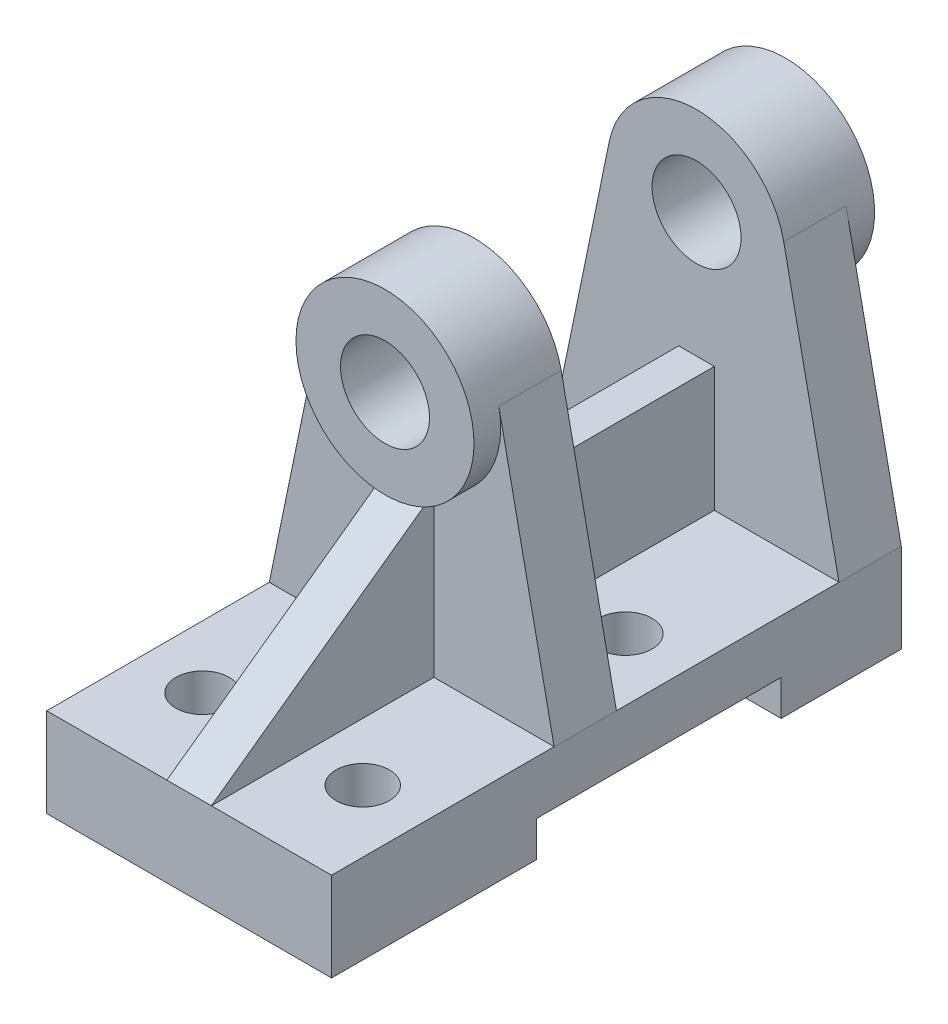
ISO-10303-21;
HEADER;
FILE_DESCRIPTION(('STEP AP214'),'2;1');
FILE_NAME('part.step','',(''),(''),'','','');
FILE_SCHEMA(('AUTOMOTIVE_DESIGN { 1 0 10303 214 1 1 1 1 }'));
ENDSEC;
DATA;
#1=APPLICATION_CONTEXT('core data for automotive mechanical design processes');
#2=APPLICATION_PROTOCOL_DEFINITION('international standard','automotive_design',2000,#1);
#3=PRODUCT_CONTEXT('',#1,'mechanical');
#4=PRODUCT('Part','Part','',(#3));
#5=PRODUCT_RELATED_PRODUCT_CATEGORY('part','',(#4));
#6=PRODUCT_DEFINITION_FORMATION('','',#4);
#7=PRODUCT_DEFINITION_CONTEXT('part definition',#1,'design');
#8=PRODUCT_DEFINITION('design','',#6,#7);
#9=PRODUCT_DEFINITION_SHAPE('','',#8);
#10=(LENGTH_UNIT() NAMED_UNIT(*) SI_UNIT(.MILLI.,.METRE.));
#11=(NAMED_UNIT(*) PLANE_ANGLE_UNIT() SI_UNIT($,.RADIAN.));
#12=(NAMED_UNIT(*) SI_UNIT($,.STERADIAN.) SOLID_ANGLE_UNIT());
#13=UNCERTAINTY_MEASURE_WITH_UNIT(LENGTH_MEASURE(1.E-05),#10,'distance_accuracy_value','');
#14=(GEOMETRIC_REPRESENTATION_CONTEXT(3) GLOBAL_UNCERTAINTY_ASSIGNED_CONTEXT((#13)) GLOBAL_UNIT_ASSIGNED_CONTEXT((#10,
#11,#12)) REPRESENTATION_CONTEXT('',''));
#15=CARTESIAN_POINT('',(0.,0.,0.));
#16=DIRECTION('',(0.,0.,1.));
#17=DIRECTION('',(1.,0.,0.));
#18=AXIS2_PLACEMENT_3D('',#15,#16,#17);
#19=CARTESIAN_POINT('',(32.,20.,0.));
#20=DIRECTION('',(0.,-1.,0.));
#21=DIRECTION('',(0.,0.,-1.));
#22=AXIS2_PLACEMENT_3D('',#19,#20,#21);
#23=PLANE('',#22);
#24=CARTESIAN_POINT('',(-18.,20.,107.));
#25=DIRECTION('',(0.,1.,0.));
#26=DIRECTION('',(0.,0.,1.));
#27=AXIS2_PLACEMENT_3D('',#24,#25,#26);
#28=CIRCLE('',#27,6.00000000000001);
#29=CARTESIAN_POINT('',(-18.,20.,113.));
#30=VERTEX_POINT('',#29);
#31=EDGE_CURVE('E600',#30,#30,#28,.T.);
#32=ORIENTED_EDGE('',*,*,#31,.F.);
#33=EDGE_LOOP('',(#32));
#34=FACE_BOUND('',#33,.T.);
#35=DIRECTION('',(0.,0.,1.));
#36=VECTOR('',#35,1.);
#37=CARTESIAN_POINT('',(-5.,20.,0.));
#38=LINE('',#37,#36);
#39=CARTESIAN_POINT('',(-5.,20.,78.));
#40=VERTEX_POINT('',#39);
#41=CARTESIAN_POINT('',(-5.,20.,128.));
#42=VERTEX_POINT('',#41);
#43=EDGE_CURVE('E215',#40,#42,#38,.T.);
#44=ORIENTED_EDGE('',*,*,#43,.F.);
#45=DIRECTION('',(1.,0.,0.));
#46=VECTOR('',#45,1.);
#47=CARTESIAN_POINT('',(0.,20.,78.));
#48=LINE('',#47,#46);
#49=CARTESIAN_POINT('',(-32.,20.,78.));
#50=VERTEX_POINT('',#49);
#51=EDGE_CURVE('E298',#50,#40,#48,.T.);
#52=ORIENTED_EDGE('',*,*,#51,.F.);
#53=DIRECTION('',(0.,0.,1.));
#54=VECTOR('',#53,1.);
#55=CARTESIAN_POINT('',(-32.,20.,0.));
#56=LINE('',#55,#54);
#57=CARTESIAN_POINT('',(-32.,20.,128.));
#58=VERTEX_POINT('',#57);
#59=EDGE_CURVE('E234',#50,#58,#56,.T.);
#60=ORIENTED_EDGE('',*,*,#59,.T.);
#61=DIRECTION('',(-1.,0.,0.));
#62=VECTOR('',#61,1.);
#63=CARTESIAN_POINT('',(32.,20.,128.));
#64=LINE('',#63,#62);
#65=EDGE_CURVE('E231',#42,#58,#64,.T.);
#66=ORIENTED_EDGE('',*,*,#65,.F.);
#67=EDGE_LOOP('',(#44,#52,#60,#66));
#68=FACE_BOUND('',#67,.T.);
#69=ADVANCED_FACE('F56',(#34,#68),#23,.F.);
#70=CARTESIAN_POINT('',(0.,0.,78.));
#71=DIRECTION('',(0.,0.,1.));
#72=DIRECTION('',(-1.,0.,0.));
#73=AXIS2_PLACEMENT_3D('',#70,#71,#72);
#74=PLANE('',#73);
#75=DIRECTION('',(0.,1.,0.));
#76=VECTOR('',#75,1.);
#77=CARTESIAN_POINT('',(5.,0.,78.));
#78=LINE('',#77,#76);
#79=CARTESIAN_POINT('',(5.,20.,78.));
#80=VERTEX_POINT('',#79);
#81=CARTESIAN_POINT('',(5.,56.,78.));
#82=VERTEX_POINT('',#81);
#83=EDGE_CURVE('E12',#80,#82,#78,.T.);
#84=ORIENTED_EDGE('',*,*,#83,.F.);
#85=CARTESIAN_POINT('',(32.,20.,78.));
#86=VERTEX_POINT('',#85);
#87=EDGE_CURVE('E294',#80,#86,#48,.T.);
#88=ORIENTED_EDGE('',*,*,#87,.T.);
#89=DIRECTION('',(0.202452606669412,-0.979292061671471,0.));
#90=VECTOR('',#89,1.);
#91=CARTESIAN_POINT('',(34.6536187572094,7.16406853737846,78.));
#92=LINE('',#91,#90);
#93=CARTESIAN_POINT('',(19.5858412334294,80.0490521333882,78.));
#94=VERTEX_POINT('',#93);
#95=EDGE_CURVE('E283',#94,#86,#92,.T.);
#96=ORIENTED_EDGE('',*,*,#95,.F.);
#97=CARTESIAN_POINT('',(0.,76.,78.));
#98=DIRECTION('',(0.,0.,1.));
#99=DIRECTION('',(1.,0.,0.));
#100=AXIS2_PLACEMENT_3D('',#97,#98,#99);
#101=CIRCLE('',#100,20.);
#102=CARTESIAN_POINT('',(0.,56.,78.));
#103=VERTEX_POINT('',#102);
#104=EDGE_CURVE('E318',#103,#94,#101,.T.);
#105=ORIENTED_EDGE('',*,*,#104,.F.);
#106=DIRECTION('',(1.,0.,0.));
#107=VECTOR('',#106,1.);
#108=CARTESIAN_POINT('',(0.,56.,78.));
#109=LINE('',#108,#107);
#110=EDGE_CURVE('E67',#82,#103,#109,.F.);
#111=ORIENTED_EDGE('',*,*,#110,.F.);
#112=EDGE_LOOP('',(#84,#88,#96,#105,#111));
#113=FACE_BOUND('',#112,.T.);
#114=ADVANCED_FACE('F430',(#113),#74,.T.);
#115=CARTESIAN_POINT('',(-18.,20.,48.));
#116=DIRECTION('',(0.,1.,0.));
#117=DIRECTION('',(0.,0.,1.));
#118=AXIS2_PLACEMENT_3D('',#115,#116,#117);
#119=CIRCLE('',#118,6.);
#120=CARTESIAN_POINT('',(-18.,20.,54.));
#121=VERTEX_POINT('',#120);
#122=EDGE_CURVE('E407',#121,#121,#119,.T.);
#123=ORIENTED_EDGE('',*,*,#122,.F.);
#124=EDGE_LOOP('',(#123));
#125=FACE_BOUND('',#124,.T.);
#126=DIRECTION('',(0.,0.,1.));
#127=VECTOR('',#126,1.);
#128=CARTESIAN_POINT('',(-4.00000000000001,20.,14.));
#129=LINE('',#128,#127);
#130=CARTESIAN_POINT('',(-4.00000000000001,20.,14.));
#131=VERTEX_POINT('',#130);
#132=CARTESIAN_POINT('',(-4.,20.,64.));
#133=VERTEX_POINT('',#132);
#134=EDGE_CURVE('E244',#131,#133,#129,.T.);
#135=ORIENTED_EDGE('',*,*,#134,.F.);
#136=DIRECTION('',(1.,0.,0.));
#137=VECTOR('',#136,1.);
#138=CARTESIAN_POINT('',(0.,20.,14.));
#139=LINE('',#138,#137);
#140=CARTESIAN_POINT('',(-32.,20.,14.));
#141=VERTEX_POINT('',#140);
#142=EDGE_CURVE('E333',#141,#131,#139,.T.);
#143=ORIENTED_EDGE('',*,*,#142,.F.);
#144=CARTESIAN_POINT('',(-32.,20.,64.));
#145=VERTEX_POINT('',#144);
#146=EDGE_CURVE('E372',#141,#145,#56,.T.);
#147=ORIENTED_EDGE('',*,*,#146,.T.);
#148=DIRECTION('',(1.,0.,0.));
#149=VECTOR('',#148,1.);
#150=CARTESIAN_POINT('',(0.,20.,64.));
#151=LINE('',#150,#149);
#152=EDGE_CURVE('E284',#145,#133,#151,.T.);
#153=ORIENTED_EDGE('',*,*,#152,.T.);
#154=EDGE_LOOP('',(#135,#143,#147,#153));
#155=FACE_BOUND('',#154,.T.);
#156=ADVANCED_FACE('F446',(#125,#155),#23,.F.);
#157=CARTESIAN_POINT('',(18.,20.,48.));
#158=DIRECTION('',(0.,1.,0.));
#159=DIRECTION('',(0.,0.,1.));
#160=AXIS2_PLACEMENT_3D('',#157,#158,#159);
#161=CIRCLE('',#160,6.);
#162=CARTESIAN_POINT('',(18.,20.,54.));
#163=VERTEX_POINT('',#162);
#164=EDGE_CURVE('E413',#163,#163,#161,.T.);
#165=ORIENTED_EDGE('',*,*,#164,.F.);
#166=EDGE_LOOP('',(#165));
#167=FACE_BOUND('',#166,.T.);
#168=DIRECTION('',(0.,0.,1.));
#169=VECTOR('',#168,1.);
#170=CARTESIAN_POINT('',(32.,20.,0.));
#171=LINE('',#170,#169);
#172=CARTESIAN_POINT('',(32.,20.,14.));
#173=VERTEX_POINT('',#172);
#174=CARTESIAN_POINT('',(32.,20.,64.));
#175=VERTEX_POINT('',#174);
#176=EDGE_CURVE('E354',#173,#175,#171,.T.);
#177=ORIENTED_EDGE('',*,*,#176,.F.);
#178=CARTESIAN_POINT('',(4.00000000000001,20.,14.));
#179=VERTEX_POINT('',#178);
#180=EDGE_CURVE('E326',#179,#173,#139,.T.);
#181=ORIENTED_EDGE('',*,*,#180,.F.);
#182=DIRECTION('',(0.,0.,-1.));
#183=VECTOR('',#182,1.);
#184=CARTESIAN_POINT('',(4.00000000000001,20.,14.));
#185=LINE('',#184,#183);
#186=CARTESIAN_POINT('',(4.,20.,64.));
#187=VERTEX_POINT('',#186);
#188=EDGE_CURVE('E250',#187,#179,#185,.T.);
#189=ORIENTED_EDGE('',*,*,#188,.F.);
#190=EDGE_CURVE('E278',#187,#175,#151,.T.);
#191=ORIENTED_EDGE('',*,*,#190,.T.);
#192=EDGE_LOOP('',(#177,#181,#189,#191));
#193=FACE_BOUND('',#192,.T.);
#194=ADVANCED_FACE('F490',(#167,#193),#23,.F.);
#195=CARTESIAN_POINT('',(0.,0.,14.));
#196=DIRECTION('',(0.,0.,-1.));
#197=DIRECTION('',(-1.,0.,0.));
#198=AXIS2_PLACEMENT_3D('',#195,#196,#197);
#199=PLANE('',#198);
#200=CARTESIAN_POINT('',(0.,76.,14.));
#201=DIRECTION('',(0.,0.,-1.));
#202=DIRECTION('',(-1.,0.,0.));
#203=AXIS2_PLACEMENT_3D('',#200,#201,#202);
#204=CIRCLE('',#203,10.);
#205=CARTESIAN_POINT('',(-10.,76.,14.));
#206=VERTEX_POINT('',#205);
#207=EDGE_CURVE('E331',#206,#206,#204,.T.);
#208=ORIENTED_EDGE('',*,*,#207,.T.);
#209=EDGE_LOOP('',(#208));
#210=FACE_BOUND('',#209,.T.);
#211=DIRECTION('',(0.202452606669412,-0.979292061671471,0.));
#212=VECTOR('',#211,1.);
#213=CARTESIAN_POINT('',(34.6536187572094,7.16406853737846,14.));
#214=LINE('',#213,#212);
#215=CARTESIAN_POINT('',(19.5858412334294,80.0490521333882,14.));
#216=VERTEX_POINT('',#215);
#217=EDGE_CURVE('E329',#216,#173,#214,.T.);
#218=ORIENTED_EDGE('',*,*,#217,.F.);
#219=CARTESIAN_POINT('',(0.,76.,14.));
#220=DIRECTION('',(0.,0.,-1.));
#221=DIRECTION('',(-1.,0.,0.));
#222=AXIS2_PLACEMENT_3D('',#219,#220,#221);
#223=CIRCLE('',#222,20.);
#224=CARTESIAN_POINT('',(-19.5858412334294,80.0490521333882,14.));
#225=VERTEX_POINT('',#224);
#226=EDGE_CURVE('E321',#225,#216,#223,.T.);
#227=ORIENTED_EDGE('',*,*,#226,.F.);
#228=DIRECTION('',(-0.202452606669412,-0.979292061671471,0.));
#229=VECTOR('',#228,1.);
#230=CARTESIAN_POINT('',(-34.6536187572094,7.16406853737846,14.));
#231=LINE('',#230,#229);
#232=EDGE_CURVE('E322',#225,#141,#231,.T.);
#233=ORIENTED_EDGE('',*,*,#232,.T.);
#234=ORIENTED_EDGE('',*,*,#142,.T.);
#235=DIRECTION('',(0.,-1.,0.));
#236=VECTOR('',#235,1.);
#237=CARTESIAN_POINT('',(-4.00000000000001,48.,14.));
#238=LINE('',#237,#236);
#239=CARTESIAN_POINT('',(-4.00000000000001,48.,14.));
#240=VERTEX_POINT('',#239);
#241=EDGE_CURVE('E256',#240,#131,#238,.T.);
#242=ORIENTED_EDGE('',*,*,#241,.F.);
#243=DIRECTION('',(-1.,0.,0.));
#244=VECTOR('',#243,1.);
#245=CARTESIAN_POINT('',(-4.00000000000001,48.,14.));
#246=LINE('',#245,#244);
#247=CARTESIAN_POINT('',(4.00000000000001,48.,14.));
#248=VERTEX_POINT('',#247);
#249=EDGE_CURVE('E259',#248,#240,#246,.T.);
#250=ORIENTED_EDGE('',*,*,#249,.F.);
#251=DIRECTION('',(0.,-1.,0.));
#252=VECTOR('',#251,1.);
#253=CARTESIAN_POINT('',(4.00000000000001,48.,14.));
#254=LINE('',#253,#252);
#255=EDGE_CURVE('E265',#248,#179,#254,.T.);
#256=ORIENTED_EDGE('',*,*,#255,.T.);
#257=ORIENTED_EDGE('',*,*,#180,.T.);
#258=EDGE_LOOP('',(#218,#227,#233,#234,#242,#250,#256,#257));
#259=FACE_BOUND('',#258,.T.);
#260=ADVANCED_FACE('F470',(#210,#259),#199,.F.);
#261=CARTESIAN_POINT('',(0.,0.,64.));
#262=DIRECTION('',(0.,0.,1.));
#263=DIRECTION('',(-1.,0.,0.));
#264=AXIS2_PLACEMENT_3D('',#261,#262,#263);
#265=PLANE('',#264);
#266=CARTESIAN_POINT('',(0.,76.,64.));
#267=DIRECTION('',(0.,0.,-1.));
#268=DIRECTION('',(-1.,0.,0.));
#269=AXIS2_PLACEMENT_3D('',#266,#267,#268);
#270=CIRCLE('',#269,10.);
#271=CARTESIAN_POINT('',(-10.,76.,64.));
#272=VERTEX_POINT('',#271);
#273=EDGE_CURVE('E287',#272,#272,#270,.T.);
#274=ORIENTED_EDGE('',*,*,#273,.F.);
#275=EDGE_LOOP('',(#274));
#276=FACE_BOUND('',#275,.T.);
#277=DIRECTION('',(0.202452606669412,-0.979292061671471,0.));
#278=VECTOR('',#277,1.);
#279=CARTESIAN_POINT('',(34.6536187572094,7.16406853737846,64.));
#280=LINE('',#279,#278);
#281=CARTESIAN_POINT('',(19.5858412334294,80.0490521333882,64.));
#282=VERTEX_POINT('',#281);
#283=EDGE_CURVE('E285',#282,#175,#280,.T.);
#284=ORIENTED_EDGE('',*,*,#283,.T.);
#285=ORIENTED_EDGE('',*,*,#190,.F.);
#286=DIRECTION('',(0.,-1.,0.));
#287=VECTOR('',#286,1.);
#288=CARTESIAN_POINT('',(4.,48.,64.));
#289=LINE('',#288,#287);
#290=CARTESIAN_POINT('',(4.,48.,64.));
#291=VERTEX_POINT('',#290);
#292=EDGE_CURVE('E270',#291,#187,#289,.T.);
#293=ORIENTED_EDGE('',*,*,#292,.F.);
#294=DIRECTION('',(1.,0.,0.));
#295=VECTOR('',#294,1.);
#296=CARTESIAN_POINT('',(-4.,48.,64.));
#297=LINE('',#296,#295);
#298=CARTESIAN_POINT('',(-4.00000000000001,48.,64.));
#299=VERTEX_POINT('',#298);
#300=EDGE_CURVE('E251',#299,#291,#297,.T.);
#301=ORIENTED_EDGE('',*,*,#300,.F.);
#302=DIRECTION('',(0.,-1.,0.));
#303=VECTOR('',#302,1.);
#304=CARTESIAN_POINT('',(-4.,48.,64.));
#305=LINE('',#304,#303);
#306=EDGE_CURVE('E81',#299,#133,#305,.T.);
#307=ORIENTED_EDGE('',*,*,#306,.T.);
#308=ORIENTED_EDGE('',*,*,#152,.F.);
#309=DIRECTION('',(-0.202452606669412,-0.979292061671471,0.));
#310=VECTOR('',#309,1.);
#311=CARTESIAN_POINT('',(-34.6536187572094,7.16406853737846,64.));
#312=LINE('',#311,#310);
#313=CARTESIAN_POINT('',(-19.5858412334294,80.0490521333882,64.));
#314=VERTEX_POINT('',#313);
#315=EDGE_CURVE('E280',#314,#145,#312,.T.);
#316=ORIENTED_EDGE('',*,*,#315,.F.);
#317=CARTESIAN_POINT('',(0.,76.,64.));
#318=DIRECTION('',(0.,0.,-1.));
#319=DIRECTION('',(-1.,0.,0.));
#320=AXIS2_PLACEMENT_3D('',#317,#318,#319);
#321=CIRCLE('',#320,20.);
#322=EDGE_CURVE('E290',#314,#282,#321,.T.);
#323=ORIENTED_EDGE('',*,*,#322,.T.);
#324=EDGE_LOOP('',(#284,#285,#293,#301,#307,#308,#316,#323));
#325=FACE_BOUND('',#324,.T.);
#326=ADVANCED_FACE('F452',(#276,#325),#265,.F.);
#327=CARTESIAN_POINT('',(18.,20.,107.));
#328=DIRECTION('',(0.,1.,0.));
#329=DIRECTION('',(0.,0.,1.));
#330=AXIS2_PLACEMENT_3D('',#327,#328,#329);
#331=CIRCLE('',#330,6.);
#332=CARTESIAN_POINT('',(18.,20.,113.));
#333=VERTEX_POINT('',#332);
#334=EDGE_CURVE('E418',#333,#333,#331,.T.);
#335=ORIENTED_EDGE('',*,*,#334,.F.);
#336=EDGE_LOOP('',(#335));
#337=FACE_BOUND('',#336,.T.);
#338=ORIENTED_EDGE('',*,*,#87,.F.);
#339=DIRECTION('',(0.,0.,1.));
#340=VECTOR('',#339,1.);
#341=CARTESIAN_POINT('',(5.,20.,0.));
#342=LINE('',#341,#340);
#343=CARTESIAN_POINT('',(5.,20.,128.));
#344=VERTEX_POINT('',#343);
#345=EDGE_CURVE('E216',#80,#344,#342,.T.);
#346=ORIENTED_EDGE('',*,*,#345,.T.);
#347=CARTESIAN_POINT('',(32.,20.,128.));
#348=VERTEX_POINT('',#347);
#349=EDGE_CURVE('E238',#348,#344,#64,.T.);
#350=ORIENTED_EDGE('',*,*,#349,.F.);
#351=EDGE_CURVE('E350',#86,#348,#171,.T.);
#352=ORIENTED_EDGE('',*,*,#351,.F.);
#353=EDGE_LOOP('',(#338,#346,#350,#352));
#354=FACE_BOUND('',#353,.T.);
#355=ADVANCED_FACE('F483',(#337,#354),#23,.F.);
#356=CARTESIAN_POINT('',(32.,0.,0.));
#357=DIRECTION('',(0.,0.,1.));
#358=DIRECTION('',(1.,0.,0.));
#359=AXIS2_PLACEMENT_3D('',#356,#357,#358);
#360=PLANE('',#359);
#361=DIRECTION('',(-1.,0.,0.));
#362=VECTOR('',#361,1.);
#363=CARTESIAN_POINT('',(32.,0.,0.));
#364=LINE('',#363,#362);
#365=CARTESIAN_POINT('',(32.,0.,0.));
#366=VERTEX_POINT('',#365);
#367=CARTESIAN_POINT('',(-32.,0.,0.));
#368=VERTEX_POINT('',#367);
#369=EDGE_CURVE('E370',#366,#368,#364,.T.);
#370=ORIENTED_EDGE('',*,*,#369,.T.);
#371=DIRECTION('',(0.,1.,0.));
#372=VECTOR('',#371,1.);
#373=CARTESIAN_POINT('',(-32.,0.,0.));
#374=LINE('',#373,#372);
#375=CARTESIAN_POINT('',(-32.,20.,0.));
#376=VERTEX_POINT('',#375);
#377=EDGE_CURVE('E341',#368,#376,#374,.T.);
#378=ORIENTED_EDGE('',*,*,#377,.T.);
#379=DIRECTION('',(-0.202452606669412,-0.979292061671471,0.));
#380=VECTOR('',#379,1.);
#381=CARTESIAN_POINT('',(-34.6536187572094,7.16406853737846,0.));
#382=LINE('',#381,#380);
#383=CARTESIAN_POINT('',(-19.5858412334294,80.0490521333882,0.));
#384=VERTEX_POINT('',#383);
#385=EDGE_CURVE('E320',#384,#376,#382,.T.);
#386=ORIENTED_EDGE('',*,*,#385,.F.);
#387=CARTESIAN_POINT('',(0.,76.,0.));
#388=DIRECTION('',(0.,0.,-1.));
#389=DIRECTION('',(-1.,0.,0.));
#390=AXIS2_PLACEMENT_3D('',#387,#388,#389);
#391=CIRCLE('',#390,20.);
#392=CARTESIAN_POINT('',(19.5858412334294,80.0490521333882,0.));
#393=VERTEX_POINT('',#392);
#394=EDGE_CURVE('E319',#393,#384,#391,.T.);
#395=ORIENTED_EDGE('',*,*,#394,.F.);
#396=DIRECTION('',(0.202452606669412,-0.979292061671471,0.));
#397=VECTOR('',#396,1.);
#398=CARTESIAN_POINT('',(34.6536187572094,7.16406853737846,0.));
#399=LINE('',#398,#397);
#400=CARTESIAN_POINT('',(32.,20.,0.));
#401=VERTEX_POINT('',#400);
#402=EDGE_CURVE('E323',#393,#401,#399,.T.);
#403=ORIENTED_EDGE('',*,*,#402,.T.);
#404=DIRECTION('',(0.,1.,0.));
#405=VECTOR('',#404,1.);
#406=CARTESIAN_POINT('',(32.,0.,0.));
#407=LINE('',#406,#405);
#408=EDGE_CURVE('E349',#366,#401,#407,.T.);
#409=ORIENTED_EDGE('',*,*,#408,.F.);
#410=EDGE_LOOP('',(#370,#378,#386,#395,#403,#409));
#411=FACE_BOUND('',#410,.T.);
#412=ADVANCED_FACE('F62',(#411),#360,.F.);
#413=CARTESIAN_POINT('',(32.,0.,128.));
#414=DIRECTION('',(0.,0.,-1.));
#415=DIRECTION('',(-1.,0.,0.));
#416=AXIS2_PLACEMENT_3D('',#413,#414,#415);
#417=PLANE('',#416);
#418=ORIENTED_EDGE('',*,*,#349,.T.);
#419=DIRECTION('',(-1.,0.,0.));
#420=VECTOR('',#419,1.);
#421=CARTESIAN_POINT('',(32.,20.,128.));
#422=LINE('',#421,#420);
#423=EDGE_CURVE('E227',#42,#344,#422,.F.);
#424=ORIENTED_EDGE('',*,*,#423,.F.);
#425=ORIENTED_EDGE('',*,*,#65,.T.);
#426=DIRECTION('',(0.,-1.,0.));
#427=VECTOR('',#426,1.);
#428=CARTESIAN_POINT('',(-32.,0.,128.));
#429=LINE('',#428,#427);
#430=CARTESIAN_POINT('',(-32.,0.,128.));
#431=VERTEX_POINT('',#430);
#432=EDGE_CURVE('E373',#58,#431,#429,.T.);
#433=ORIENTED_EDGE('',*,*,#432,.T.);
#434=DIRECTION('',(-1.,0.,0.));
#435=VECTOR('',#434,1.);
#436=CARTESIAN_POINT('',(32.,0.,128.));
#437=LINE('',#436,#435);
#438=CARTESIAN_POINT('',(32.,0.,128.));
#439=VERTEX_POINT('',#438);
#440=EDGE_CURVE('E237',#439,#431,#437,.T.);
#441=ORIENTED_EDGE('',*,*,#440,.F.);
#442=DIRECTION('',(0.,-1.,0.));
#443=VECTOR('',#442,1.);
#444=CARTESIAN_POINT('',(32.,0.,128.));
#445=LINE('',#444,#443);
#446=EDGE_CURVE('E352',#348,#439,#445,.T.);
#447=ORIENTED_EDGE('',*,*,#446,.F.);
#448=EDGE_LOOP('',(#418,#424,#425,#433,#441,#447));
#449=FACE_BOUND('',#448,.T.);
#450=ADVANCED_FACE('F245',(#449),#417,.F.);
#451=CARTESIAN_POINT('',(32.,0.,82.));
#452=DIRECTION('',(0.,1.,0.));
#453=DIRECTION('',(0.,0.,1.));
#454=AXIS2_PLACEMENT_3D('',#451,#452,#453);
#455=PLANE('',#454);
#456=CARTESIAN_POINT('',(-18.,0.,107.));
#457=DIRECTION('',(0.,1.,0.));
#458=DIRECTION('',(0.,0.,1.));
#459=AXIS2_PLACEMENT_3D('',#456,#457,#458);
#460=CIRCLE('',#459,6.00000000000001);
#461=CARTESIAN_POINT('',(-18.,0.,113.));
#462=VERTEX_POINT('',#461);
#463=EDGE_CURVE('E419',#462,#462,#460,.T.);
#464=ORIENTED_EDGE('',*,*,#463,.T.);
#465=EDGE_LOOP('',(#464));
#466=FACE_BOUND('',#465,.T.);
#467=CARTESIAN_POINT('',(18.,0.,107.));
#468=DIRECTION('',(0.,1.,0.));
#469=DIRECTION('',(0.,0.,1.));
#470=AXIS2_PLACEMENT_3D('',#467,#468,#469);
#471=CIRCLE('',#470,6.);
#472=CARTESIAN_POINT('',(18.,0.,113.));
#473=VERTEX_POINT('',#472);
#474=EDGE_CURVE('E596',#473,#473,#471,.T.);
#475=ORIENTED_EDGE('',*,*,#474,.T.);
#476=EDGE_LOOP('',(#475));
#477=FACE_BOUND('',#476,.T.);
#478=ORIENTED_EDGE('',*,*,#440,.T.);
#479=DIRECTION('',(0.,0.,-1.));
#480=VECTOR('',#479,1.);
#481=CARTESIAN_POINT('',(-32.,0.,82.));
#482=LINE('',#481,#480);
#483=CARTESIAN_POINT('',(-32.,0.,82.));
#484=VERTEX_POINT('',#483);
#485=EDGE_CURVE('E376',#431,#484,#482,.T.);
#486=ORIENTED_EDGE('',*,*,#485,.T.);
#487=DIRECTION('',(-1.,0.,0.));
#488=VECTOR('',#487,1.);
#489=CARTESIAN_POINT('',(32.,0.,82.));
#490=LINE('',#489,#488);
#491=CARTESIAN_POINT('',(32.,0.,82.));
#492=VERTEX_POINT('',#491);
#493=EDGE_CURVE('E400',#492,#484,#490,.T.);
#494=ORIENTED_EDGE('',*,*,#493,.F.);
#495=DIRECTION('',(0.,0.,-1.));
#496=VECTOR('',#495,1.);
#497=CARTESIAN_POINT('',(32.,0.,82.));
#498=LINE('',#497,#496);
#499=EDGE_CURVE('E357',#439,#492,#498,.T.);
#500=ORIENTED_EDGE('',*,*,#499,.F.);
#501=EDGE_LOOP('',(#478,#486,#494,#500));
#502=FACE_BOUND('',#501,.T.);
#503=ADVANCED_FACE('F551',(#466,#477,#502),#455,.F.);
#504=CARTESIAN_POINT('',(32.,0.,82.));
#505=DIRECTION('',(0.,0.,1.));
#506=DIRECTION('',(0.,-1.,0.));
#507=AXIS2_PLACEMENT_3D('',#504,#505,#506);
#508=PLANE('',#507);
#509=ORIENTED_EDGE('',*,*,#493,.T.);
#510=DIRECTION('',(0.,1.,0.));
#511=VECTOR('',#510,1.);
#512=CARTESIAN_POINT('',(-32.,0.,82.));
#513=LINE('',#512,#511);
#514=CARTESIAN_POINT('',(-32.,7.99999999999999,82.));
#515=VERTEX_POINT('',#514);
#516=EDGE_CURVE('E378',#484,#515,#513,.T.);
#517=ORIENTED_EDGE('',*,*,#516,.T.);
#518=DIRECTION('',(-1.,0.,0.));
#519=VECTOR('',#518,1.);
#520=CARTESIAN_POINT('',(32.,7.99999999999999,82.));
#521=LINE('',#520,#519);
#522=CARTESIAN_POINT('',(32.,7.99999999999999,82.));
#523=VERTEX_POINT('',#522);
#524=EDGE_CURVE('E391',#523,#515,#521,.T.);
#525=ORIENTED_EDGE('',*,*,#524,.F.);
#526=DIRECTION('',(0.,1.,0.));
#527=VECTOR('',#526,1.);
#528=CARTESIAN_POINT('',(32.,0.,82.));
#529=LINE('',#528,#527);
#530=EDGE_CURVE('E360',#492,#523,#529,.T.);
#531=ORIENTED_EDGE('',*,*,#530,.F.);
#532=EDGE_LOOP('',(#509,#517,#525,#531));
#533=FACE_BOUND('',#532,.T.);
#534=ADVANCED_FACE('F546',(#533),#508,.F.);
#535=CARTESIAN_POINT('',(32.,8.,27.));
#536=DIRECTION('',(0.,1.,0.));
#537=DIRECTION('',(0.,0.,1.));
#538=AXIS2_PLACEMENT_3D('',#535,#536,#537);
#539=PLANE('',#538);
#540=CARTESIAN_POINT('',(18.,7.99999999999999,48.));
#541=DIRECTION('',(0.,1.,0.));
#542=DIRECTION('',(0.,0.,1.));
#543=AXIS2_PLACEMENT_3D('',#540,#541,#542);
#544=CIRCLE('',#543,6.);
#545=CARTESIAN_POINT('',(18.,7.99999999999999,54.));
#546=VERTEX_POINT('',#545);
#547=EDGE_CURVE('E64',#546,#546,#544,.T.);
#548=ORIENTED_EDGE('',*,*,#547,.T.);
#549=EDGE_LOOP('',(#548));
#550=FACE_BOUND('',#549,.T.);
#551=CARTESIAN_POINT('',(-18.,7.99999999999999,48.));
#552=DIRECTION('',(0.,1.,0.));
#553=DIRECTION('',(0.,0.,1.));
#554=AXIS2_PLACEMENT_3D('',#551,#552,#553);
#555=CIRCLE('',#554,6.);
#556=CARTESIAN_POINT('',(-18.,7.99999999999999,54.));
#557=VERTEX_POINT('',#556);
#558=EDGE_CURVE('E404',#557,#557,#555,.T.);
#559=ORIENTED_EDGE('',*,*,#558,.T.);
#560=EDGE_LOOP('',(#559));
#561=FACE_BOUND('',#560,.T.);
#562=ORIENTED_EDGE('',*,*,#524,.T.);
#563=DIRECTION('',(0.,0.,-1.));
#564=VECTOR('',#563,1.);
#565=CARTESIAN_POINT('',(-32.,8.,27.));
#566=LINE('',#565,#564);
#567=CARTESIAN_POINT('',(-32.,8.,27.));
#568=VERTEX_POINT('',#567);
#569=EDGE_CURVE('E385',#515,#568,#566,.T.);
#570=ORIENTED_EDGE('',*,*,#569,.T.);
#571=DIRECTION('',(-1.,0.,0.));
#572=VECTOR('',#571,1.);
#573=CARTESIAN_POINT('',(32.,8.,27.));
#574=LINE('',#573,#572);
#575=CARTESIAN_POINT('',(32.,8.,27.));
#576=VERTEX_POINT('',#575);
#577=EDGE_CURVE('E392',#576,#568,#574,.T.);
#578=ORIENTED_EDGE('',*,*,#577,.F.);
#579=DIRECTION('',(0.,0.,-1.));
#580=VECTOR('',#579,1.);
#581=CARTESIAN_POINT('',(32.,8.,27.));
#582=LINE('',#581,#580);
#583=EDGE_CURVE('E363',#523,#576,#582,.T.);
#584=ORIENTED_EDGE('',*,*,#583,.F.);
#585=EDGE_LOOP('',(#562,#570,#578,#584));
#586=FACE_BOUND('',#585,.T.);
#587=ADVANCED_FACE('F542',(#550,#561,#586),#539,.F.);
#588=CARTESIAN_POINT('',(32.,0.,27.));
#589=DIRECTION('',(0.,0.,-1.));
#590=DIRECTION('',(0.,1.,0.));
#591=AXIS2_PLACEMENT_3D('',#588,#589,#590);
#592=PLANE('',#591);
#593=ORIENTED_EDGE('',*,*,#577,.T.);
#594=DIRECTION('',(0.,-1.,0.));
#595=VECTOR('',#594,1.);
#596=CARTESIAN_POINT('',(-32.,0.,27.));
#597=LINE('',#596,#595);
#598=CARTESIAN_POINT('',(-32.,0.,27.));
#599=VERTEX_POINT('',#598);
#600=EDGE_CURVE('E383',#568,#599,#597,.T.);
#601=ORIENTED_EDGE('',*,*,#600,.T.);
#602=DIRECTION('',(-1.,0.,0.));
#603=VECTOR('',#602,1.);
#604=CARTESIAN_POINT('',(32.,0.,27.));
#605=LINE('',#604,#603);
#606=CARTESIAN_POINT('',(32.,0.,27.));
#607=VERTEX_POINT('',#606);
#608=EDGE_CURVE('E393',#607,#599,#605,.T.);
#609=ORIENTED_EDGE('',*,*,#608,.F.);
#610=DIRECTION('',(0.,-1.,0.));
#611=VECTOR('',#610,1.);
#612=CARTESIAN_POINT('',(32.,0.,27.));
#613=LINE('',#612,#611);
#614=EDGE_CURVE('E361',#576,#607,#613,.T.);
#615=ORIENTED_EDGE('',*,*,#614,.F.);
#616=EDGE_LOOP('',(#593,#601,#609,#615));
#617=FACE_BOUND('',#616,.T.);
#618=ADVANCED_FACE('F536',(#617),#592,.F.);
#619=CARTESIAN_POINT('',(32.,0.,0.));
#620=DIRECTION('',(0.,1.,0.));
#621=DIRECTION('',(0.,0.,1.));
#622=AXIS2_PLACEMENT_3D('',#619,#620,#621);
#623=PLANE('',#622);
#624=ORIENTED_EDGE('',*,*,#608,.T.);
#625=DIRECTION('',(0.,0.,-1.));
#626=VECTOR('',#625,1.);
#627=CARTESIAN_POINT('',(-32.,0.,0.));
#628=LINE('',#627,#626);
#629=EDGE_CURVE('E346',#599,#368,#628,.T.);
#630=ORIENTED_EDGE('',*,*,#629,.T.);
#631=ORIENTED_EDGE('',*,*,#369,.F.);
#632=DIRECTION('',(0.,0.,-1.));
#633=VECTOR('',#632,1.);
#634=CARTESIAN_POINT('',(32.,0.,0.));
#635=LINE('',#634,#633);
#636=EDGE_CURVE('E362',#607,#366,#635,.T.);
#637=ORIENTED_EDGE('',*,*,#636,.F.);
#638=EDGE_LOOP('',(#624,#630,#631,#637));
#639=FACE_BOUND('',#638,.T.);
#640=ADVANCED_FACE('F533',(#639),#623,.F.);
#641=CARTESIAN_POINT('',(32.,0.,0.));
#642=DIRECTION('',(1.,0.,0.));
#643=DIRECTION('',(0.,0.,-1.));
#644=AXIS2_PLACEMENT_3D('',#641,#642,#643);
#645=PLANE('',#644);
#646=ORIENTED_EDGE('',*,*,#408,.T.);
#647=EDGE_CURVE('E353',#401,#173,#171,.T.);
#648=ORIENTED_EDGE('',*,*,#647,.T.);
#649=ORIENTED_EDGE('',*,*,#176,.T.);
#650=DIRECTION('',(0.,0.,1.));
#651=VECTOR('',#650,1.);
#652=CARTESIAN_POINT('',(32.,20.,64.));
#653=LINE('',#652,#651);
#654=EDGE_CURVE('E310',#175,#86,#653,.T.);
#655=ORIENTED_EDGE('',*,*,#654,.T.);
#656=ORIENTED_EDGE('',*,*,#351,.T.);
#657=ORIENTED_EDGE('',*,*,#446,.T.);
#658=ORIENTED_EDGE('',*,*,#499,.T.);
#659=ORIENTED_EDGE('',*,*,#530,.T.);
#660=ORIENTED_EDGE('',*,*,#583,.T.);
#661=ORIENTED_EDGE('',*,*,#614,.T.);
#662=ORIENTED_EDGE('',*,*,#636,.T.);
#663=EDGE_LOOP('',(#646,#648,#649,#655,#656,#657,#658,#659,#660,#661,#662));
#664=FACE_BOUND('',#663,.T.);
#665=ADVANCED_FACE('F518',(#664),#645,.T.);
#666=CARTESIAN_POINT('',(-32.,0.,0.));
#667=DIRECTION('',(1.,0.,0.));
#668=DIRECTION('',(0.,0.,-1.));
#669=AXIS2_PLACEMENT_3D('',#666,#667,#668);
#670=PLANE('',#669);
#671=ORIENTED_EDGE('',*,*,#377,.F.);
#672=ORIENTED_EDGE('',*,*,#629,.F.);
#673=ORIENTED_EDGE('',*,*,#600,.F.);
#674=ORIENTED_EDGE('',*,*,#569,.F.);
#675=ORIENTED_EDGE('',*,*,#516,.F.);
#676=ORIENTED_EDGE('',*,*,#485,.F.);
#677=ORIENTED_EDGE('',*,*,#432,.F.);
#678=ORIENTED_EDGE('',*,*,#59,.F.);
#679=DIRECTION('',(0.,0.,1.));
#680=VECTOR('',#679,1.);
#681=CARTESIAN_POINT('',(-32.,20.,64.));
#682=LINE('',#681,#680);
#683=EDGE_CURVE('E292',#145,#50,#682,.T.);
#684=ORIENTED_EDGE('',*,*,#683,.F.);
#685=ORIENTED_EDGE('',*,*,#146,.F.);
#686=EDGE_CURVE('E369',#376,#141,#56,.T.);
#687=ORIENTED_EDGE('',*,*,#686,.F.);
#688=EDGE_LOOP('',(#671,#672,#673,#674,#675,#676,#677,#678,#684,#685,#687));
#689=FACE_BOUND('',#688,.T.);
#690=ADVANCED_FACE('F444',(#689),#670,.F.);
#691=CARTESIAN_POINT('',(-34.6536187572094,7.16406853737846,14.));
#692=DIRECTION('',(0.979292061671471,-0.202452606669412,0.));
#693=DIRECTION('',(0.202452606669412,0.979292061671471,0.));
#694=AXIS2_PLACEMENT_3D('',#691,#692,#693);
#695=PLANE('',#694);
#696=ORIENTED_EDGE('',*,*,#385,.T.);
#697=ORIENTED_EDGE('',*,*,#686,.T.);
#698=ORIENTED_EDGE('',*,*,#232,.F.);
#699=DIRECTION('',(0.,0.,-1.));
#700=VECTOR('',#699,1.);
#701=CARTESIAN_POINT('',(-19.5858412334294,80.0490521333882,14.));
#702=LINE('',#701,#700);
#703=EDGE_CURVE('E337',#225,#384,#702,.T.);
#704=ORIENTED_EDGE('',*,*,#703,.T.);
#705=EDGE_LOOP('',(#696,#697,#698,#704));
#706=FACE_BOUND('',#705,.T.);
#707=ADVANCED_FACE('F529',(#706),#695,.F.);
#708=CARTESIAN_POINT('',(34.6536187572094,7.16406853737846,14.));
#709=DIRECTION('',(0.979292061671471,0.202452606669412,0.));
#710=DIRECTION('',(-0.202452606669412,0.979292061671471,0.));
#711=AXIS2_PLACEMENT_3D('',#708,#709,#710);
#712=PLANE('',#711);
#713=ORIENTED_EDGE('',*,*,#402,.F.);
#714=DIRECTION('',(0.,0.,-1.));
#715=VECTOR('',#714,1.);
#716=CARTESIAN_POINT('',(19.5858412334294,80.0490521333882,14.));
#717=LINE('',#716,#715);
#718=EDGE_CURVE('E342',#216,#393,#717,.T.);
#719=ORIENTED_EDGE('',*,*,#718,.F.);
#720=ORIENTED_EDGE('',*,*,#217,.T.);
#721=ORIENTED_EDGE('',*,*,#647,.F.);
#722=EDGE_LOOP('',(#713,#719,#720,#721));
#723=FACE_BOUND('',#722,.T.);
#724=ADVANCED_FACE('F519',(#723),#712,.T.);
#725=CARTESIAN_POINT('',(0.,76.,14.));
#726=DIRECTION('',(0.,0.,-1.));
#727=DIRECTION('',(-1.,0.,0.));
#728=AXIS2_PLACEMENT_3D('',#725,#726,#727);
#729=CYLINDRICAL_SURFACE('',#728,20.);
#730=ORIENTED_EDGE('',*,*,#394,.T.);
#731=ORIENTED_EDGE('',*,*,#703,.F.);
#732=ORIENTED_EDGE('',*,*,#226,.T.);
#733=ORIENTED_EDGE('',*,*,#718,.T.);
#734=EDGE_LOOP('',(#730,#731,#732,#733));
#735=FACE_BOUND('',#734,.T.);
#736=CARTESIAN_POINT('',(0.,76.,-6.));
#737=DIRECTION('',(0.,0.,-1.));
#738=DIRECTION('',(-1.,0.,0.));
#739=AXIS2_PLACEMENT_3D('',#736,#737,#738);
#740=CIRCLE('',#739,20.);
#741=CARTESIAN_POINT('',(-20.,76.,-6.));
#742=VERTEX_POINT('',#741);
#743=EDGE_CURVE('E313',#742,#742,#740,.T.);
#744=ORIENTED_EDGE('',*,*,#743,.F.);
#745=EDGE_LOOP('',(#744));
#746=FACE_BOUND('',#745,.T.);
#747=ADVANCED_FACE('F528',(#735,#746),#729,.T.);
#748=CARTESIAN_POINT('',(0.,76.,14.));
#749=DIRECTION('',(0.,0.,-1.));
#750=DIRECTION('',(-1.,0.,0.));
#751=AXIS2_PLACEMENT_3D('',#748,#749,#750);
#752=CYLINDRICAL_SURFACE('',#751,10.);
#753=ORIENTED_EDGE('',*,*,#207,.F.);
#754=EDGE_LOOP('',(#753));
#755=FACE_BOUND('',#754,.T.);
#756=CARTESIAN_POINT('',(0.,76.,-6.));
#757=DIRECTION('',(0.,0.,-1.));
#758=DIRECTION('',(-1.,0.,0.));
#759=AXIS2_PLACEMENT_3D('',#756,#757,#758);
#760=CIRCLE('',#759,10.);
#761=CARTESIAN_POINT('',(-10.,76.,-6.));
#762=VERTEX_POINT('',#761);
#763=EDGE_CURVE('E303',#762,#762,#760,.T.);
#764=ORIENTED_EDGE('',*,*,#763,.T.);
#765=EDGE_LOOP('',(#764));
#766=FACE_BOUND('',#765,.T.);
#767=ADVANCED_FACE('F629',(#755,#766),#752,.F.);
#768=CARTESIAN_POINT('',(0.,76.,-6.));
#769=DIRECTION('',(0.,0.,-1.));
#770=DIRECTION('',(-1.,0.,0.));
#771=AXIS2_PLACEMENT_3D('',#768,#769,#770);
#772=PLANE('',#771);
#773=ORIENTED_EDGE('',*,*,#763,.F.);
#774=EDGE_LOOP('',(#773));
#775=FACE_BOUND('',#774,.T.);
#776=ORIENTED_EDGE('',*,*,#743,.T.);
#777=EDGE_LOOP('',(#776));
#778=FACE_BOUND('',#777,.T.);
#779=ADVANCED_FACE('F632',(#775,#778),#772,.T.);
#780=CARTESIAN_POINT('',(-34.6536187572094,7.16406853737846,64.));
#781=DIRECTION('',(-0.979292061671471,0.202452606669412,0.));
#782=DIRECTION('',(-0.202452606669412,-0.979292061671471,0.));
#783=AXIS2_PLACEMENT_3D('',#780,#781,#782);
#784=PLANE('',#783);
#785=DIRECTION('',(-0.202452606669412,-0.979292061671471,0.));
#786=VECTOR('',#785,1.);
#787=CARTESIAN_POINT('',(-34.6536187572094,7.16406853737846,78.));
#788=LINE('',#787,#786);
#789=CARTESIAN_POINT('',(-19.5858412334294,80.0490521333882,78.));
#790=VERTEX_POINT('',#789);
#791=EDGE_CURVE('E277',#790,#50,#788,.T.);
#792=ORIENTED_EDGE('',*,*,#791,.F.);
#793=DIRECTION('',(0.,0.,1.));
#794=VECTOR('',#793,1.);
#795=CARTESIAN_POINT('',(-19.5858412334294,80.0490521333882,64.));
#796=LINE('',#795,#794);
#797=EDGE_CURVE('E297',#314,#790,#796,.T.);
#798=ORIENTED_EDGE('',*,*,#797,.F.);
#799=ORIENTED_EDGE('',*,*,#315,.T.);
#800=ORIENTED_EDGE('',*,*,#683,.T.);
#801=EDGE_LOOP('',(#792,#798,#799,#800));
#802=FACE_BOUND('',#801,.T.);
#803=ADVANCED_FACE('F437',(#802),#784,.T.);
#804=CARTESIAN_POINT('',(0.,76.,64.));
#805=DIRECTION('',(0.,0.,1.));
#806=DIRECTION('',(1.,0.,0.));
#807=AXIS2_PLACEMENT_3D('',#804,#805,#806);
#808=CYLINDRICAL_SURFACE('',#807,20.);
#809=ORIENTED_EDGE('',*,*,#797,.T.);
#810=EDGE_CURVE('E399',#790,#103,#101,.T.);
#811=ORIENTED_EDGE('',*,*,#810,.T.);
#812=ORIENTED_EDGE('',*,*,#104,.T.);
#813=DIRECTION('',(0.,0.,1.));
#814=VECTOR('',#813,1.);
#815=CARTESIAN_POINT('',(19.5858412334294,80.0490521333882,64.));
#816=LINE('',#815,#814);
#817=EDGE_CURVE('E302',#282,#94,#816,.T.);
#818=ORIENTED_EDGE('',*,*,#817,.F.);
#819=ORIENTED_EDGE('',*,*,#322,.F.);
#820=EDGE_LOOP('',(#809,#811,#812,#818,#819));
#821=FACE_BOUND('',#820,.T.);
#822=CARTESIAN_POINT('',(0.,76.,84.));
#823=DIRECTION('',(0.,0.,-1.));
#824=DIRECTION('',(-1.,0.,0.));
#825=AXIS2_PLACEMENT_3D('',#822,#823,#824);
#826=CIRCLE('',#825,20.);
#827=CARTESIAN_POINT('',(-20.,76.,84.));
#828=VERTEX_POINT('',#827);
#829=EDGE_CURVE('E271',#828,#828,#826,.T.);
#830=ORIENTED_EDGE('',*,*,#829,.T.);
#831=EDGE_LOOP('',(#830));
#832=FACE_BOUND('',#831,.T.);
#833=ADVANCED_FACE('F435',(#821,#832),#808,.T.);
#834=CARTESIAN_POINT('',(34.6536187572094,7.16406853737846,64.));
#835=DIRECTION('',(-0.979292061671471,-0.202452606669412,0.));
#836=DIRECTION('',(0.202452606669412,-0.979292061671471,0.));
#837=AXIS2_PLACEMENT_3D('',#834,#835,#836);
#838=PLANE('',#837);
#839=ORIENTED_EDGE('',*,*,#95,.T.);
#840=ORIENTED_EDGE('',*,*,#654,.F.);
#841=ORIENTED_EDGE('',*,*,#283,.F.);
#842=ORIENTED_EDGE('',*,*,#817,.T.);
#843=EDGE_LOOP('',(#839,#840,#841,#842));
#844=FACE_BOUND('',#843,.T.);
#845=ADVANCED_FACE('F645',(#844),#838,.F.);
#846=CARTESIAN_POINT('',(0.,76.,64.));
#847=DIRECTION('',(0.,0.,1.));
#848=DIRECTION('',(1.,0.,0.));
#849=AXIS2_PLACEMENT_3D('',#846,#847,#848);
#850=CYLINDRICAL_SURFACE('',#849,10.);
#851=ORIENTED_EDGE('',*,*,#273,.T.);
#852=EDGE_LOOP('',(#851));
#853=FACE_BOUND('',#852,.T.);
#854=CARTESIAN_POINT('',(0.,76.,84.));
#855=DIRECTION('',(0.,0.,-1.));
#856=DIRECTION('',(-1.,0.,0.));
#857=AXIS2_PLACEMENT_3D('',#854,#855,#856);
#858=CIRCLE('',#857,10.);
#859=CARTESIAN_POINT('',(-10.,76.,84.));
#860=VERTEX_POINT('',#859);
#861=EDGE_CURVE('E269',#860,#860,#858,.T.);
#862=ORIENTED_EDGE('',*,*,#861,.F.);
#863=EDGE_LOOP('',(#862));
#864=FACE_BOUND('',#863,.T.);
#865=ADVANCED_FACE('F643',(#853,#864),#850,.F.);
#866=CARTESIAN_POINT('',(-5.,56.,78.));
#867=VERTEX_POINT('',#866);
#868=EDGE_CURVE('E229',#103,#867,#109,.F.);
#869=ORIENTED_EDGE('',*,*,#868,.F.);
#870=ORIENTED_EDGE('',*,*,#810,.F.);
#871=ORIENTED_EDGE('',*,*,#791,.T.);
#872=ORIENTED_EDGE('',*,*,#51,.T.);
#873=DIRECTION('',(0.,1.,0.));
#874=VECTOR('',#873,1.);
#875=CARTESIAN_POINT('',(-5.,0.,78.));
#876=LINE('',#875,#874);
#877=EDGE_CURVE('E213',#40,#867,#876,.T.);
#878=ORIENTED_EDGE('',*,*,#877,.T.);
#879=EDGE_LOOP('',(#869,#870,#871,#872,#878));
#880=FACE_BOUND('',#879,.T.);
#881=ADVANCED_FACE('F440',(#880),#74,.T.);
#882=CARTESIAN_POINT('',(0.,76.,84.));
#883=DIRECTION('',(0.,0.,1.));
#884=DIRECTION('',(-1.,0.,0.));
#885=AXIS2_PLACEMENT_3D('',#882,#883,#884);
#886=PLANE('',#885);
#887=ORIENTED_EDGE('',*,*,#861,.T.);
#888=EDGE_LOOP('',(#887));
#889=FACE_BOUND('',#888,.T.);
#890=ORIENTED_EDGE('',*,*,#829,.F.);
#891=EDGE_LOOP('',(#890));
#892=FACE_BOUND('',#891,.T.);
#893=ADVANCED_FACE('F468',(#889,#892),#886,.T.);
#894=CARTESIAN_POINT('',(-4.00000000000001,48.,14.));
#895=DIRECTION('',(1.,0.,0.));
#896=DIRECTION('',(0.,0.,-1.));
#897=AXIS2_PLACEMENT_3D('',#894,#895,#896);
#898=PLANE('',#897);
#899=ORIENTED_EDGE('',*,*,#134,.T.);
#900=ORIENTED_EDGE('',*,*,#306,.F.);
#901=DIRECTION('',(0.,0.,1.));
#902=VECTOR('',#901,1.);
#903=CARTESIAN_POINT('',(-4.00000000000001,48.,14.));
#904=LINE('',#903,#902);
#905=EDGE_CURVE('E255',#240,#299,#904,.T.);
#906=ORIENTED_EDGE('',*,*,#905,.F.);
#907=ORIENTED_EDGE('',*,*,#241,.T.);
#908=EDGE_LOOP('',(#899,#900,#906,#907));
#909=FACE_BOUND('',#908,.T.);
#910=ADVANCED_FACE('F466',(#909),#898,.F.);
#911=CARTESIAN_POINT('',(4.00000000000001,48.,14.));
#912=DIRECTION('',(-1.,0.,0.));
#913=DIRECTION('',(0.,0.,1.));
#914=AXIS2_PLACEMENT_3D('',#911,#912,#913);
#915=PLANE('',#914);
#916=ORIENTED_EDGE('',*,*,#188,.T.);
#917=ORIENTED_EDGE('',*,*,#255,.F.);
#918=DIRECTION('',(0.,0.,-1.));
#919=VECTOR('',#918,1.);
#920=CARTESIAN_POINT('',(4.00000000000001,48.,14.));
#921=LINE('',#920,#919);
#922=EDGE_CURVE('E257',#291,#248,#921,.T.);
#923=ORIENTED_EDGE('',*,*,#922,.F.);
#924=ORIENTED_EDGE('',*,*,#292,.T.);
#925=EDGE_LOOP('',(#916,#917,#923,#924));
#926=FACE_BOUND('',#925,.T.);
#927=ADVANCED_FACE('F456',(#926),#915,.F.);
#928=CARTESIAN_POINT('',(0.,48.,0.));
#929=DIRECTION('',(0.,1.,0.));
#930=DIRECTION('',(0.,0.,1.));
#931=AXIS2_PLACEMENT_3D('',#928,#929,#930);
#932=PLANE('',#931);
#933=ORIENTED_EDGE('',*,*,#905,.T.);
#934=ORIENTED_EDGE('',*,*,#300,.T.);
#935=ORIENTED_EDGE('',*,*,#922,.T.);
#936=ORIENTED_EDGE('',*,*,#249,.T.);
#937=EDGE_LOOP('',(#933,#934,#935,#936));
#938=FACE_BOUND('',#937,.T.);
#939=ADVANCED_FACE('F459',(#938),#932,.T.);
#940=CARTESIAN_POINT('',(5.,48.,61.));
#941=DIRECTION('',(1.,0.,0.));
#942=DIRECTION('',(0.,0.,-1.));
#943=AXIS2_PLACEMENT_3D('',#940,#941,#942);
#944=PLANE('',#943);
#945=ORIENTED_EDGE('',*,*,#345,.F.);
#946=ORIENTED_EDGE('',*,*,#83,.T.);
#947=DIRECTION('',(0.,0.584304725845076,-0.811534341451494));
#948=VECTOR('',#947,1.);
#949=CARTESIAN_POINT('',(5.,20.,128.));
#950=LINE('',#949,#948);
#951=EDGE_CURVE('E223',#344,#82,#950,.T.);
#952=ORIENTED_EDGE('',*,*,#951,.F.);
#953=EDGE_LOOP('',(#945,#946,#952));
#954=FACE_BOUND('',#953,.T.);
#955=ADVANCED_FACE('F560',(#954),#944,.T.);
#956=CARTESIAN_POINT('',(-5.,48.,61.));
#957=DIRECTION('',(1.,0.,0.));
#958=DIRECTION('',(0.,0.,-1.));
#959=AXIS2_PLACEMENT_3D('',#956,#957,#958);
#960=PLANE('',#959);
#961=ORIENTED_EDGE('',*,*,#877,.F.);
#962=ORIENTED_EDGE('',*,*,#43,.T.);
#963=DIRECTION('',(0.,0.584304725845076,-0.811534341451494));
#964=VECTOR('',#963,1.);
#965=CARTESIAN_POINT('',(-5.,20.,128.));
#966=LINE('',#965,#964);
#967=EDGE_CURVE('E77',#42,#867,#966,.T.);
#968=ORIENTED_EDGE('',*,*,#967,.T.);
#969=EDGE_LOOP('',(#961,#962,#968));
#970=FACE_BOUND('',#969,.T.);
#971=ADVANCED_FACE('F214',(#970),#960,.F.);
#972=CARTESIAN_POINT('',(0.,20.,128.));
#973=DIRECTION('',(0.,-0.811534341451494,-0.584304725845076));
#974=DIRECTION('',(0.,0.584304725845076,-0.811534341451494));
#975=AXIS2_PLACEMENT_3D('',#972,#973,#974);
#976=PLANE('',#975);
#977=ORIENTED_EDGE('',*,*,#967,.F.);
#978=ORIENTED_EDGE('',*,*,#423,.T.);
#979=ORIENTED_EDGE('',*,*,#951,.T.);
#980=ORIENTED_EDGE('',*,*,#110,.T.);
#981=ORIENTED_EDGE('',*,*,#868,.T.);
#982=EDGE_LOOP('',(#977,#978,#979,#980,#981));
#983=FACE_BOUND('',#982,.T.);
#984=ADVANCED_FACE('F222',(#983),#976,.F.);
#985=CARTESIAN_POINT('',(-18.,0.,48.));
#986=DIRECTION('',(0.,1.,0.));
#987=DIRECTION('',(0.,0.,1.));
#988=AXIS2_PLACEMENT_3D('',#985,#986,#987);
#989=CYLINDRICAL_SURFACE('',#988,6.);
#990=ORIENTED_EDGE('',*,*,#122,.T.);
#991=EDGE_LOOP('',(#990));
#992=FACE_BOUND('',#991,.T.);
#993=ORIENTED_EDGE('',*,*,#558,.F.);
#994=EDGE_LOOP('',(#993));
#995=FACE_BOUND('',#994,.T.);
#996=ADVANCED_FACE('F570',(#992,#995),#989,.F.);
#997=CARTESIAN_POINT('',(18.,0.,48.));
#998=DIRECTION('',(0.,1.,0.));
#999=DIRECTION('',(0.,0.,1.));
#1000=AXIS2_PLACEMENT_3D('',#997,#998,#999);
#1001=CYLINDRICAL_SURFACE('',#1000,6.);
#1002=ORIENTED_EDGE('',*,*,#164,.T.);
#1003=EDGE_LOOP('',(#1002));
#1004=FACE_BOUND('',#1003,.T.);
#1005=ORIENTED_EDGE('',*,*,#547,.F.);
#1006=EDGE_LOOP('',(#1005));
#1007=FACE_BOUND('',#1006,.T.);
#1008=ADVANCED_FACE('F573',(#1004,#1007),#1001,.F.);
#1009=CARTESIAN_POINT('',(18.,0.,107.));
#1010=DIRECTION('',(0.,1.,0.));
#1011=DIRECTION('',(0.,0.,1.));
#1012=AXIS2_PLACEMENT_3D('',#1009,#1010,#1011);
#1013=CYLINDRICAL_SURFACE('',#1012,6.);
#1014=ORIENTED_EDGE('',*,*,#474,.F.);
#1015=EDGE_LOOP('',(#1014));
#1016=FACE_BOUND('',#1015,.T.);
#1017=ORIENTED_EDGE('',*,*,#334,.T.);
#1018=EDGE_LOOP('',(#1017));
#1019=FACE_BOUND('',#1018,.T.);
#1020=ADVANCED_FACE('F579',(#1016,#1019),#1013,.F.);
#1021=CARTESIAN_POINT('',(-18.,0.,107.));
#1022=DIRECTION('',(0.,1.,0.));
#1023=DIRECTION('',(0.,0.,1.));
#1024=AXIS2_PLACEMENT_3D('',#1021,#1022,#1023);
#1025=CYLINDRICAL_SURFACE('',#1024,6.00000000000001);
#1026=ORIENTED_EDGE('',*,*,#463,.F.);
#1027=EDGE_LOOP('',(#1026));
#1028=FACE_BOUND('',#1027,.T.);
#1029=ORIENTED_EDGE('',*,*,#31,.T.);
#1030=EDGE_LOOP('',(#1029));
#1031=FACE_BOUND('',#1030,.T.);
#1032=ADVANCED_FACE('F583',(#1028,#1031),#1025,.F.);
#1033=CLOSED_SHELL('',(#69,#114,#156,#194,#260,#326,#355,#412,#450,#503,#534,#587,#618,#640,
#665,#690,#707,#724,#747,#767,#779,#803,#833,#845,#865,#881,#893,#910,#927,#939,#955,#971,#984,
#996,#1008,#1020,#1032));
#1034=MANIFOLD_SOLID_BREP('B2',#1033);
#1035=ADVANCED_BREP_SHAPE_REPRESENTATION('',(#18,#1034),#14);
#1036=SHAPE_DEFINITION_REPRESENTATION(#9,#1035);
ENDSEC;
END-ISO-10303-21;
